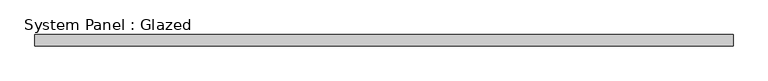
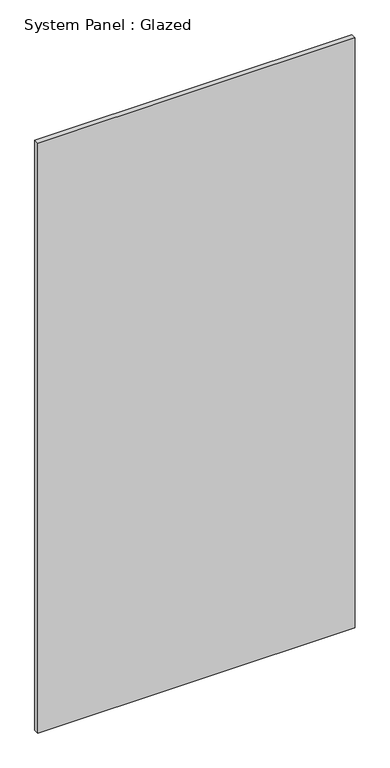
"""IFC4 building model written with IfcOpenShell, lengths in millimetres: plate geometry, System Panel : Glazed."""

from ifc_helpers import new_model, si_unit, origin, origin_with_axes, place, context, project, spatial, polyline, outline, extrude, source, transform, mapped, element, save


def system_panel_glazed_557224e7(model_context):
    return source(origin(), model_context, "Body", "SweptSolid", [
        extrude(outline(polyline([(763.632, 24.5), (-763.632, 24.5), (-763.632, 49.5), (763.632, 49.5), (763.632, 24.5)])), origin_with_axes(), (0.0, 0.0, 1.0), 3000.0),
    ])


if __name__ == "__main__":
    model = new_model("IFC4")
    model_context = context("Model", 3, world=origin())
    ifc_project = project(units=[si_unit("LENGTHUNIT", "METRE", prefix="MILLI")], contexts=[model_context])
    site = spatial("IfcSite", under=ifc_project)
    building = spatial("IfcBuilding", under=site)
    placement = place(None, origin())
    system_panel_glazed_shape = system_panel_glazed_557224e7(model_context)
    element("IfcPlate", 1, ObjectType="System Panel : Glazed", at=placement, inside=building, context=model_context, shape_type="MappedRepresentation", body=[
        mapped(system_panel_glazed_shape, transform((0.0, 0.0, 0.0), x_axis=(1.0, 0.0, 0.0), y_axis=(0.0, 1.0, 0.0), z_axis=(0.0, 0.0, 1.0))),
    ])
    save(model, "model.ifc")

# Revit data of these elements
# Type "System Panel : Glazed"
#   Keynote = "H11"
#   Construction Type Id = "GSP4R"
#   Analytic Construction = "1/8 in Pilkington single glazing"
#   Visual Light Transmittance = 0.9
#   Solar Heat Gain Coefficient = 0.86
#   Heat Transfer Coefficient (U) = 6.7069 W/(m²·K)
#   Define Thermal Properties by = 1
# Element 1 (IfcPlate, "System Panel : Glazed")
#   Materials on its faces: "Glass"
# Materials
#   "Glass": class "Glass", colour RGB 0 128 192, transparency 0.9, Description = "Soda Lime Glass", Cost = 0
